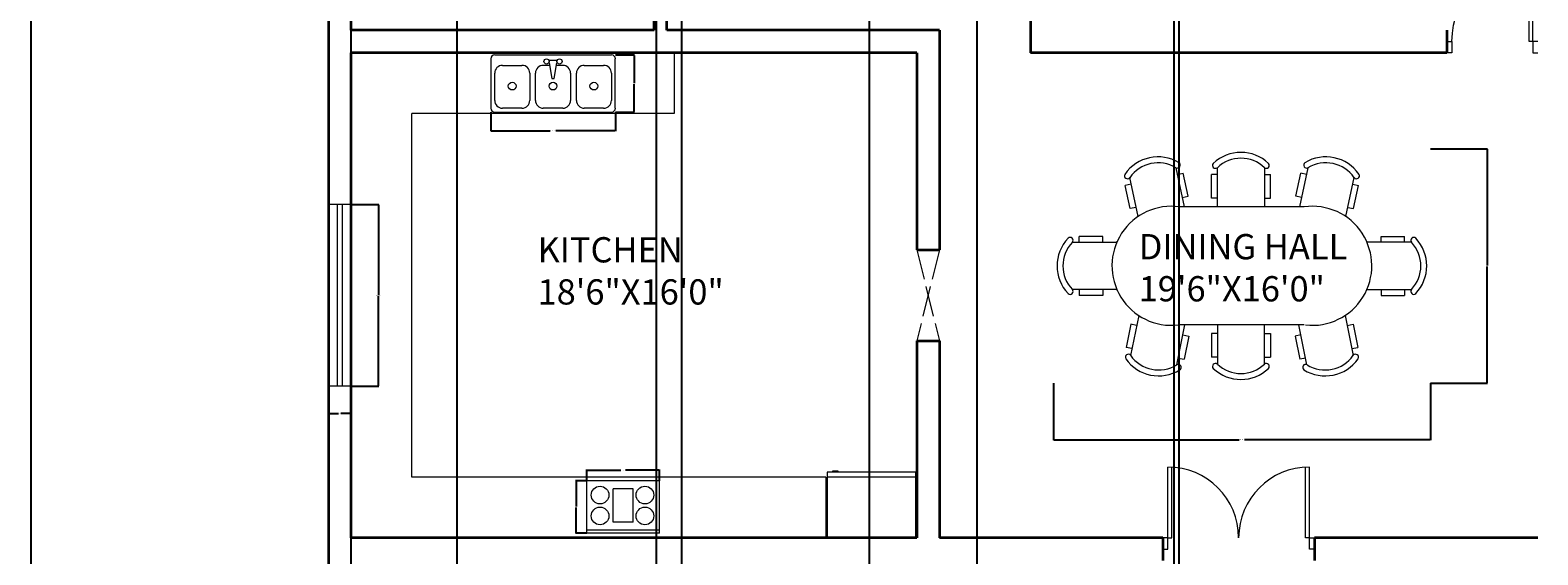
# Model space of a CAD drawing. Units: inches. Extents: x 4602 to 5612, y 5125 to 6591.
# Tile 4 of 6: x 4602 to 5199, y 5977 to 6185. Entities that reach past the tile are written whole.
import ezdxf

# ---------------------------------------------------------------- set-up
doc = ezdxf.new("R2010")
doc.units = ezdxf.units.IN
doc.linetypes.add('ACAD_ISO02W100', pattern=[15, 12, -3])
for name, color, linetype, lineweight in [('A-ANNO-DIMS', 2, 'Continuous', 18), ('A-AREA-IDEN', 7, 'Continuous', 18), ('A-DOOR', 4, 'Continuous', 18), ('A-EQPM', 8, 'Continuous', 18), ('A-FLOR-CASE', 9, 'Continuous', 18), ('A-FLOR-FIXT', 8, 'Continuous', 18), ('A-FURN', 8, 'Continuous', 13), ('A-GLAZ', 4, 'Continuous', 18), ('A-WALL', 7, 'Continuous', 35), ('A-WALL-OVHD', 8, 'ACAD_ISO02W100', 13)]:
    doc.layers.add(name, color=color, linetype=linetype, lineweight=lineweight)
doc.styles.get("Standard").update_dxf_attribs({"font": 'arial.ttf'})
doc.dimstyles.get("Standard").update_dxf_attribs({"dimtxt": 0.18, "dimasz": 0.18, "dimexe": 0.18, "dimexo": 0.0625, "dimgap": 0.09, "dimtad": 0, "dimtih": 1, "dimtoh": 1, "dimdec": 4, "dimzin": 0, "dimdsep": 46, "dimtxsty": 'Standard', "dimcen": 0.09, "dimadec": 0, "dimazin": 0, "dimtfac": 1, "dimtdec": 4, "dimtofl": 0, "dimtmove": 0, "dimatfit": 3, "dimfxl": 1, "dimtolj": 1, "dimtzin": 0, "dimarcsym": 0})

# ---------------------------------------------------------------- blocks, each defined once
blk = doc.blocks.new('A$C47C54457')
for p, q in [((0, 520), (720, 520)), ((0, 520), (0, 0)), ((0, 488), (720, 488)), ((720, 520), (720, 0)), ((262, 408), (458, 408)), ((262, 408), (262, 80)), ((458, 408), (458, 80)), ((0, 0), (720, 0)), ((262, 80), (458, 80))]:
    blk.add_line(p, q)
for centre in [(144, 348), (590, 348), (144, 140), (590, 140)]:
    blk.add_circle(centre, 88)
blk = doc.blocks.new('A$C4CC12AE8')
for p, q in [((1.006, 1.792), (1.077, 1.461)), ((1.357, 1.461), (1.357, 1.792)), ((1.757, 1.792), (1.757, 1.461)), ((2.124, 1.792), (2.053, 1.461)), ((0.686, 1.378), (0.615, 1.708)), ((1.018, 1.736), (1.067, 1.746)), ((1.109, 1.55), (1.067, 1.746)), ((1.357, 1.734), (1.307, 1.734)), ((1.307, 1.534), (1.307, 1.734)), ((1.757, 1.734), (1.807, 1.734)), ((1.807, 1.534), (1.807, 1.734)), ((2.022, 1.55), (2.063, 1.746)), ((2.112, 1.736), (2.063, 1.746)), ((2.445, 1.378), (2.515, 1.708)), ((0.627, 1.652), (0.578, 1.641)), ((0.62, 1.446), (0.578, 1.641)), ((1.06, 1.54), (1.109, 1.55)), ((1.357, 1.534), (1.307, 1.534)), ((1.757, 1.534), (1.807, 1.534)), ((2.07, 1.54), (2.022, 1.55)), ((2.503, 1.652), (2.552, 1.641)), ((2.51, 1.446), (2.552, 1.641)), ((0.669, 1.456), (0.62, 1.446)), ((2.093, 1.461), (1.038, 1.461)), ((2.462, 1.456), (2.51, 1.446)), ((0.13, 1.161), (0.5, 1.161)), ((0.188, 1.161), (0.188, 1.211)), ((0.388, 1.211), (0.188, 1.211)), ((0.388, 1.161), (0.388, 1.211)), ((3.001, 1.161), (2.631, 1.161)), ((2.743, 1.161), (2.743, 1.211)), ((2.743, 1.211), (2.943, 1.211)), ((2.943, 1.161), (2.943, 1.211)), ((0.5, 0.761), (0.13, 0.761)), ((0.188, 0.761), (0.188, 0.711)), ((0.388, 0.711), (0.188, 0.711)), ((0.388, 0.761), (0.388, 0.711)), ((2.631, 0.761), (3.001, 0.761)), ((2.743, 0.761), (2.743, 0.711)), ((2.743, 0.711), (2.943, 0.711)), ((2.943, 0.761), (2.943, 0.711)), ((0.691, 0.542), (0.622, 0.204)), ((2.439, 0.542), (2.508, 0.204)), ((0.625, 0.467), (0.585, 0.271)), ((0.674, 0.457), (0.625, 0.467)), ((1.014, 0.124), (1.083, 0.461)), ((2.093, 0.461), (1.038, 0.461)), ((1.357, 0.388), (1.307, 0.388)), ((1.307, 0.388), (1.307, 0.188)), ((1.357, 0.461), (1.357, 0.13)), ((1.757, 0.13), (1.757, 0.461)), ((1.757, 0.388), (1.807, 0.388)), ((1.807, 0.388), (1.807, 0.188)), ((2.116, 0.124), (2.048, 0.461)), ((2.457, 0.457), (2.506, 0.467)), ((2.506, 0.467), (2.546, 0.271)), ((0.634, 0.261), (0.585, 0.271)), ((1.066, 0.377), (1.115, 0.367)), ((1.115, 0.367), (1.075, 0.171)), ((2.065, 0.377), (2.016, 0.367)), ((2.016, 0.367), (2.056, 0.171)), ((2.497, 0.261), (2.546, 0.271)), ((1.026, 0.181), (1.075, 0.171)), ((1.357, 0.188), (1.307, 0.188)), ((1.757, 0.188), (1.807, 0.188)), ((2.105, 0.181), (2.056, 0.171))]:
    blk.add_line(p, q)
for centre, radius, start, end in [((1.557, 1.582), 0.34, 46.4394, 133.5606), ((0.855, 1.544), 0.34, 58.5263, 145.6476), ((0.855, 1.544), 0.29, 58.5263, 145.6476), ((1.017, 1.814), 0.0251, 243.3074, 53.7452), ((1.341, 1.812), 0.0251, 138.3417, 308.7795), ((1.557, 1.582), 0.29, 46.4394, 133.5606), ((1.772, 1.812), 0.0251, 231.2205, 41.6583), ((2.113, 1.814), 0.0251, 126.2548, 296.6926), ((2.276, 1.544), 0.34, 34.3524, 121.4737), ((2.276, 1.544), 0.29, 34.3524, 121.4737), ((0.596, 1.724), 0.0251, 150.4287, 320.8665), ((2.535, 1.724), 0.0251, 219.1335, 29.5713), ((0.969, 0.962), 0.504, 82.2325, 276.4385), ((2.161, 0.962), 0.504, 263.5615, 97.7675), ((0.34, 0.961), 0.34, 136.4394, 223.5606), ((0.34, 0.961), 0.29, 136.4394, 223.5606), ((0.11, 1.177), 0.0251, 321.2205, 131.6583), ((0.5, 1.131), 0.03, 77.6511, 90), ((2.631, 1.131), 0.03, 90, 102.3489), ((3.02, 1.177), 0.0251, 48.3417, 218.7795), ((2.79, 0.961), 0.29, 316.4394, 43.5606), ((2.79, 0.961), 0.34, 316.4394, 43.5606), ((0.11, 0.745), 0.0251, 228.3417, 38.7795), ((0.5, 0.791), 0.03, 270, 283.3086), ((2.631, 0.791), 0.03, 256.6914, 270), ((3.02, 0.745), 0.0251, 141.2205, 311.6583), ((0.603, 0.188), 0.0251, 39.6982, 210.136), ((0.86, 0.37), 0.34, 214.9171, 302.0384), ((0.86, 0.37), 0.29, 214.9171, 302.0384), ((1.341, 0.11), 0.0251, 51.2205, 221.6583), ((1.557, 0.34), 0.29, 226.4394, 313.5606), ((1.772, 0.11), 0.0251, 318.3417, 128.7795), ((2.27, 0.37), 0.34, 237.9616, 325.0829), ((2.27, 0.37), 0.29, 237.9616, 325.0829), ((2.527, 0.188), 0.0251, 329.864, 140.3018), ((1.026, 0.102), 0.0251, 306.8195, 117.2573), ((1.557, 0.34), 0.34, 226.4394, 313.5606), ((2.105, 0.102), 0.0251, 62.7427, 233.1805)]:
    blk.add_arc(centre, radius, start, end)
blk = doc.blocks.new('A$C762E1B96')
at = {"linetype": 'ByBlock'}
for p, q in [((0, 420), (0, 31)), ((952, 450), (31, 450)), ((92, 368), (246, 368)), ((464, 368), (414, 368)), ((460, 409), (522, 409)), ((460, 389), (481, 266)), ((501, 266), (522, 389)), ((568, 368), (518, 368)), ((737, 368), (890, 368)), ((982, 31), (982, 420)), ((31, 92), (31, 307)), ((307, 307), (307, 92)), ((353, 92), (353, 307)), ((481, 266), (501, 266)), ((629, 307), (629, 92)), ((675, 92), (675, 307)), ((952, 307), (952, 92)), ((246, 31), (92, 31)), ((568, 31), (414, 31)), ((890, 31), (737, 31)), ((31, 0), (952, 0))]:
    blk.add_line(p, q, dxfattribs=at)
for centre, radius in [((440, 399), 20.5), ((542, 399), 20.5), ((169, 205), 30.7), ((491, 205), 30.7), ((813, 205), 30.7)]:
    blk.add_circle(centre, radius, dxfattribs=at)
for centre, radius, start, end in [((31, 420), 30.7, 90, 180), ((92, 307), 61.4, 90, 180), ((246, 307), 61.4, 0, 90), ((414, 307), 61.4, 90, 180), ((568, 307), 61.4, 0, 90), ((737, 307), 61.4, 90, 180), ((890, 307), 61.4, 0, 90), ((952, 420), 30.7, 0, 90), ((31, 31), 30.7, 180, 270), ((92, 92), 61.4, 180, 270), ((246, 92), 61.4, 270, 0), ((414, 92), 61.4, 180, 270), ((568, 92), 61.4, 270, 0), ((737, 92), 61.4, 180, 270), ((890, 92), 61.4, 270, 0), ((952, 31), 30.7, 270, 0)]:
    blk.add_arc(centre, radius, start, end, dxfattribs=at)
at = {"flags": 9}
for tag in ['YSIZE', 'XSIZE']:
    blk.add_attdef(tag, (491, 450), '', height=0.5, rotation=270, dxfattribs=at)
blk = doc.blocks.new('DOOR-PAIR-60IN')
for p, q in [((2, 4.5), (2, 32.5)), ((3.5, 4.5), (3.5, 32.46)), ((56.5, 4.5), (56.5, 32.46)), ((58, 4.5), (58, 32.5)), ((2, 4.5), (0, 4.5)), ((2, 0), (2, 4.5)), ((2, 4.5), (3.5, 4.5)), ((58, 4.5), (56.5, 4.5)), ((58, 0), (58, 4.5)), ((58, 4.5), (60, 4.5)), ((0, 0), (2, 0)), ((60, 0), (58, 0))]:
    blk.add_line(p, q)
for centre, start, end in [((2, 4.5), 0, 90), ((58, 4.5), 90, 180)]:
    blk.add_arc(centre, 28, start, end)
blk = doc.blocks.new('DOOR-36IN-DEEP-JAMB')
for p, q in [((2, 4.5), (2, 36.5)), ((3.5, 4.5), (3.5, 36.46)), ((0, 4.5), (2, 4.5)), ((2, 4.5), (2, 0)), ((2, 4.5), (3.5, 4.5)), ((36, 4.5), (34, 4.5)), ((34, 4.5), (34, 0)), ((2, 0), (0, 0)), ((34, 0), (36, 0))]:
    blk.add_line(p, q)
blk.add_arc((2, 4.5), 32, 0, 90)
blk = doc.blocks.new('WINDOW-72IN')
for p, q in [((9, 72), (0, 72)), ((3.5, 72), (3.5, 0)), ((5.5, 72), (5.5, 0)), ((9, 0), (0, 0))]:
    blk.add_line(p, q)
blk = doc.blocks.new('*D31')
at = {"layer": 'A-ANNO-DIMS', "color": 0, "lineweight": -2, "transparency": 16777216}
for p, q in [((4729.3, 6115.55), (4740.22, 6115.55)), ((4740.04, 6115.37), (4740.04, 6079.73)), ((4740.04, 6043.73), (4740.04, 6079.37)), ((4729.3, 6043.55), (4740.22, 6043.55))]:
    blk.add_line(p, q, dxfattribs=at)
at = {"layer": 'A-ANNO-DIMS', "color": 0, "transparency": 16777216}
for points in [[(4740.01, 6115.37), (4740.07, 6115.37), (4740.04, 6115.55)], [(4740.01, 6043.73), (4740.07, 6043.73), (4740.04, 6043.55)]]:
    blk.add_solid(points, dxfattribs=at)
at = {"layer": 'Defpoints', "color": 0, "transparency": 16777216}
for p in [(4729.24, 6115.55), (4740.04, 6115.55), (4729.24, 6043.55)]:
    blk.add_point(p, dxfattribs=at)
at = {"layer": 'A-ANNO-DIMS', "color": 0, "transparency": 16777216, "insert": (4740.04, 6079.55), "char_height": 0.18, "attachment_point": 5}
blk.add_mtext('\\A1;WINDOW 72 TYP.', dxfattribs=at)
blk = doc.blocks.new('*D32')
at = {"layer": 'A-ANNO-DIMS', "color": 0, "lineweight": -2, "transparency": 16777216}
for p, q in [((4720.24, 6043.49), (4720.24, 6032.57)), ((4729.24, 6043.49), (4729.24, 6032.57)), ((4720.42, 6032.75), (4724.28, 6032.75)), ((4729.06, 6032.75), (4725.2, 6032.75))]:
    blk.add_line(p, q, dxfattribs=at)
at = {"layer": 'A-ANNO-DIMS', "color": 0, "transparency": 16777216}
for points in [[(4720.42, 6032.78), (4720.42, 6032.72), (4720.24, 6032.75)], [(4729.06, 6032.78), (4729.06, 6032.72), (4729.24, 6032.75)]]:
    blk.add_solid(points, dxfattribs=at)
at = {"layer": 'Defpoints', "color": 0, "transparency": 16777216}
for p in [(4720.24, 6043.55), (4729.24, 6043.55), (4729.24, 6032.75)]:
    blk.add_point(p, dxfattribs=at)
at = {"layer": 'A-ANNO-DIMS', "color": 0, "transparency": 16777216, "insert": (4724.74, 6032.75), "char_height": 0.18, "attachment_point": 5}
blk.add_mtext('\\A1;9 TYP.', dxfattribs=at)
blk = doc.blocks.new('*D45')
at = {"layer": 'A-ANNO-DIMS', "color": 0, "lineweight": -2, "transparency": 16777216}
for p, q in [((4822.63, 6006.13), (4822.63, 6010.55)), ((4822.81, 6010.37), (4836.11, 6010.37)), ((4851.16, 6010.37), (4837.87, 6010.37)), ((4851.34, 6006.13), (4851.34, 6010.55))]:
    blk.add_line(p, q, dxfattribs=at)
at = {"layer": 'A-ANNO-DIMS', "color": 0, "transparency": 16777216}
for points in [[(4822.81, 6010.4), (4822.81, 6010.34), (4822.63, 6010.37)], [(4851.16, 6010.4), (4851.16, 6010.34), (4851.34, 6010.37)]]:
    blk.add_solid(points, dxfattribs=at)
at = {"layer": 'Defpoints', "color": 0, "transparency": 16777216}
for p in [(4822.63, 6010.37), (4822.63, 6006.06), (4851.34, 6006.06)]:
    blk.add_point(p, dxfattribs=at)
at = {"layer": 'A-ANNO-DIMS', "color": 0, "transparency": 16777216, "insert": (4836.99, 6010.37), "char_height": 0.18, "attachment_point": 5}
blk.add_mtext('\\A1;COOKTOP 29', dxfattribs=at)
blk = doc.blocks.new('*D46')
at = {"layer": 'A-ANNO-DIMS', "color": 0, "lineweight": -2, "transparency": 16777216}
for p, q in [((4822.57, 6006.06), (4818.15, 6006.06)), ((4818.33, 6005.88), (4818.33, 5995.88)), ((4818.33, 5985.51), (4818.33, 5995.52)), ((4822.57, 5985.33), (4818.15, 5985.33))]:
    blk.add_line(p, q, dxfattribs=at)
at = {"layer": 'A-ANNO-DIMS', "color": 0, "transparency": 16777216}
for points in [[(4818.3, 6005.88), (4818.36, 6005.88), (4818.33, 6006.06)], [(4818.3, 5985.51), (4818.36, 5985.51), (4818.33, 5985.33)]]:
    blk.add_solid(points, dxfattribs=at)
at = {"layer": 'Defpoints', "color": 0, "transparency": 16777216}
for p in [(4822.63, 6006.06), (4818.33, 5985.33), (4822.63, 5985.33)]:
    blk.add_point(p, dxfattribs=at)
at = {"layer": 'A-ANNO-DIMS', "color": 0, "transparency": 16777216, "insert": (4818.33, 5995.7), "char_height": 0.18, "attachment_point": 5}
blk.add_mtext('\\A1;21', dxfattribs=at)
blk = doc.blocks.new('*D47')
at = {"layer": 'A-ANNO-DIMS', "color": 0, "lineweight": -2, "transparency": 16777216}
for p, q in [((5007.36, 6044.73), (5007.36, 6022.21)), ((5156.72, 6044.73), (5156.72, 6022.21)), ((5007.54, 6022.39), (5081, 6022.39)), ((5156.54, 6022.39), (5083.08, 6022.39))]:
    blk.add_line(p, q, dxfattribs=at)
at = {"layer": 'A-ANNO-DIMS', "color": 0, "transparency": 16777216}
for points in [[(5007.54, 6022.42), (5007.54, 6022.36), (5007.36, 6022.39)], [(5156.54, 6022.42), (5156.54, 6022.36), (5156.72, 6022.39)]]:
    blk.add_solid(points, dxfattribs=at)
at = {"layer": 'Defpoints', "color": 0, "transparency": 16777216}
for p in [(5007.36, 6044.79), (5156.72, 6044.79), (5156.72, 6022.39)]:
    blk.add_point(p, dxfattribs=at)
at = {"layer": 'A-ANNO-DIMS', "color": 0, "transparency": 16777216, "insert": (5082.04, 6022.39), "char_height": 0.18, "attachment_point": 5}
blk.add_mtext('\\A1;DINING SET 149', dxfattribs=at)
blk = doc.blocks.new('*D48')
at = {"layer": 'A-ANNO-DIMS', "color": 0, "lineweight": -2, "transparency": 16777216}
for p, q in [((5156.78, 6137.62), (5179.3, 6137.62)), ((5179.12, 6137.44), (5179.12, 6091.39)), ((5179.12, 6044.97), (5179.12, 6091.02)), ((5156.78, 6044.79), (5179.3, 6044.79))]:
    blk.add_line(p, q, dxfattribs=at)
at = {"layer": 'A-ANNO-DIMS', "color": 0, "transparency": 16777216}
for points in [[(5179.09, 6137.44), (5179.15, 6137.44), (5179.12, 6137.62)], [(5179.09, 6044.97), (5179.15, 6044.97), (5179.12, 6044.79)]]:
    blk.add_solid(points, dxfattribs=at)
at = {"layer": 'Defpoints', "color": 0, "transparency": 16777216}
for p in [(5156.72, 6137.62), (5179.12, 6137.62), (5156.72, 6044.79)]:
    blk.add_point(p, dxfattribs=at)
at = {"layer": 'A-ANNO-DIMS', "color": 0, "transparency": 16777216, "insert": (5179.12, 6091.21), "char_height": 0.18, "attachment_point": 5}
blk.add_mtext('\\A1;93', dxfattribs=at)
blk = doc.blocks.new('*D53')
at = {"layer": 'A-ANNO-DIMS', "color": 0, "lineweight": -2, "transparency": 16777216}
for p, q in [((4784.55, 6152.05), (4784.55, 6144.53)), ((4833.89, 6152.05), (4833.89, 6144.53)), ((4784.73, 6144.71), (4808.09, 6144.71)), ((4833.71, 6144.71), (4810.35, 6144.71))]:
    blk.add_line(p, q, dxfattribs=at)
at = {"layer": 'A-ANNO-DIMS', "color": 0, "transparency": 16777216}
for points in [[(4784.73, 6144.74), (4784.73, 6144.68), (4784.55, 6144.71)], [(4833.71, 6144.74), (4833.71, 6144.68), (4833.89, 6144.71)]]:
    blk.add_solid(points, dxfattribs=at)
at = {"layer": 'Defpoints', "color": 0, "transparency": 16777216}
for p in [(4784.55, 6152.11), (4833.89, 6152.11), (4833.89, 6144.71)]:
    blk.add_point(p, dxfattribs=at)
at = {"layer": 'A-ANNO-DIMS', "color": 0, "transparency": 16777216, "insert": (4809.22, 6144.71), "char_height": 0.18, "attachment_point": 5}
blk.add_mtext('\\A1;KITCHEN SINK 49', dxfattribs=at)
blk = doc.blocks.new('*D54')
at = {"layer": 'A-ANNO-DIMS', "color": 0, "lineweight": -2, "transparency": 16777216}
for p, q in [((4833.95, 6174.72), (4841.47, 6174.72)), ((4841.29, 6174.54), (4841.29, 6163.6)), ((4841.29, 6152.29), (4841.29, 6163.23)), ((4833.95, 6152.11), (4841.47, 6152.11))]:
    blk.add_line(p, q, dxfattribs=at)
at = {"layer": 'A-ANNO-DIMS', "color": 0, "transparency": 16777216}
for points in [[(4841.26, 6174.54), (4841.32, 6174.54), (4841.29, 6174.72)], [(4841.26, 6152.29), (4841.32, 6152.29), (4841.29, 6152.11)]]:
    blk.add_solid(points, dxfattribs=at)
at = {"layer": 'Defpoints', "color": 0, "transparency": 16777216}
for p in [(4833.89, 6174.72), (4841.29, 6174.72), (4833.89, 6152.11)]:
    blk.add_point(p, dxfattribs=at)
at = {"layer": 'A-ANNO-DIMS', "color": 0, "transparency": 16777216, "insert": (4841.29, 6163.41), "char_height": 0.18, "attachment_point": 5}
blk.add_mtext('\\A1;23', dxfattribs=at)
blk = doc.blocks.new('*D55')
at = {"layer": 'A-ANNO-DIMS', "color": 0, "lineweight": -2, "transparency": 16777216}
for p, q in [((4674.24, 6252.95), (4674.24, 6572.85)), ((4674.42, 6572.67), (5106.95, 6572.67)), ((5540.06, 6572.67), (5107.53, 6572.67)), ((5540.24, 6127.61), (5540.24, 6572.85))]:
    blk.add_line(p, q, dxfattribs=at)
at = {"layer": 'A-ANNO-DIMS', "color": 0, "transparency": 16777216}
for points in [[(4674.42, 6572.7), (4674.42, 6572.64), (4674.24, 6572.67)], [(5540.06, 6572.7), (5540.06, 6572.64), (5540.24, 6572.67)]]:
    blk.add_solid(points, dxfattribs=at)
at = {"layer": 'Defpoints', "color": 0, "transparency": 16777216}
for p in [(5540.24, 6572.67), (4674.24, 6252.89), (5540.24, 6127.55)]:
    blk.add_point(p, dxfattribs=at)
at = {"layer": 'A-ANNO-DIMS', "color": 0, "transparency": 16777216, "insert": (5107.24, 6572.67), "char_height": 0.18, "attachment_point": 5}
blk.add_mtext('\\A1;866', dxfattribs=at)
blk = doc.blocks.new('*D56')
at = {"layer": 'A-ANNO-DIMS', "color": 0, "lineweight": -2, "transparency": 16777216}
for p, q in [((5061.18, 6438.55), (4602.21, 6438.55)), ((4602.39, 6438.37), (4602.39, 5817.73)), ((4602.39, 5196.73), (4602.39, 5817.37)), ((5055.18, 5196.55), (4602.21, 5196.55))]:
    blk.add_line(p, q, dxfattribs=at)
at = {"layer": 'A-ANNO-DIMS', "color": 0, "transparency": 16777216}
for points in [[(4602.36, 6438.37), (4602.42, 6438.37), (4602.39, 6438.55)], [(4602.36, 5196.73), (4602.42, 5196.73), (4602.39, 5196.55)]]:
    blk.add_solid(points, dxfattribs=at)
at = {"layer": 'Defpoints', "color": 0, "transparency": 16777216}
for p in [(4602.39, 6438.55), (5061.24, 6438.55), (5055.24, 5196.55)]:
    blk.add_point(p, dxfattribs=at)
at = {"layer": 'A-ANNO-DIMS', "color": 0, "transparency": 16777216, "insert": (4602.39, 5817.55), "char_height": 0.18, "attachment_point": 5}
blk.add_mtext('\\A1;1242', dxfattribs=at)
blk = doc.blocks.new('*D59')
at = {"layer": 'A-ANNO-DIMS', "color": 0, "lineweight": -2, "transparency": 16777216}
for p, q in [((4977.24, 5908.61), (4977.24, 6572.85)), ((4977.42, 6572.67), (5016.82, 6572.67)), ((5056.97, 6572.67), (5017.57, 6572.67)), ((5057.15, 5908.61), (5057.15, 6572.85))]:
    blk.add_line(p, q, dxfattribs=at)
at = {"layer": 'A-ANNO-DIMS', "color": 0, "transparency": 16777216}
for points in [[(4977.42, 6572.7), (4977.42, 6572.64), (4977.24, 6572.67)], [(5056.97, 6572.7), (5056.97, 6572.64), (5057.15, 6572.67)]]:
    blk.add_solid(points, dxfattribs=at)
at = {"layer": 'Defpoints', "color": 0, "transparency": 16777216}
for p in [(5057.15, 6572.67), (4977.24, 5908.55), (5057.15, 5908.55)]:
    blk.add_point(p, dxfattribs=at)
at = {"layer": 'A-ANNO-DIMS', "color": 0, "transparency": 16777216, "insert": (5017.19, 6572.67), "char_height": 0.18, "attachment_point": 5}
blk.add_mtext('\\A1;79.91', dxfattribs=at)
blk = doc.blocks.new('*D60')
at = {"layer": 'A-ANNO-DIMS', "color": 0, "lineweight": -2, "transparency": 16777216}
for p, q in [((4934.59, 5248.61), (4934.59, 6572.85)), ((4934.77, 6572.67), (4994.46, 6572.67)), ((5055.06, 6572.67), (4995.37, 6572.67)), ((5055.24, 5248.61), (5055.24, 6572.85))]:
    blk.add_line(p, q, dxfattribs=at)
at = {"layer": 'A-ANNO-DIMS', "color": 0, "transparency": 16777216}
for points in [[(4934.77, 6572.7), (4934.77, 6572.64), (4934.59, 6572.67)], [(5055.06, 6572.7), (5055.06, 6572.64), (5055.24, 6572.67)]]:
    blk.add_solid(points, dxfattribs=at)
at = {"layer": 'Defpoints', "color": 0, "transparency": 16777216}
for p in [(5055.24, 6572.67), (4934.59, 5248.55), (5055.24, 5248.55)]:
    blk.add_point(p, dxfattribs=at)
at = {"layer": 'A-ANNO-DIMS', "color": 0, "transparency": 16777216, "insert": (4994.91, 6572.67), "char_height": 0.18, "attachment_point": 5}
blk.add_mtext('\\A1;120.65', dxfattribs=at)
blk = doc.blocks.new('*D62')
at = {"layer": 'A-ANNO-DIMS', "color": 0, "lineweight": -2, "transparency": 16777216}
for p, q in [((4729.24, 5886.61), (4729.24, 6572.85)), ((4729.42, 6572.67), (4750.02, 6572.67)), ((4771.06, 6572.67), (4750.46, 6572.67)), ((4771.24, 5886.61), (4771.24, 6572.85))]:
    blk.add_line(p, q, dxfattribs=at)
at = {"layer": 'A-ANNO-DIMS', "color": 0, "transparency": 16777216}
for points in [[(4729.42, 6572.7), (4729.42, 6572.64), (4729.24, 6572.67)], [(4771.06, 6572.7), (4771.06, 6572.64), (4771.24, 6572.67)]]:
    blk.add_solid(points, dxfattribs=at)
at = {"layer": 'Defpoints', "color": 0, "transparency": 16777216}
for p in [(4771.24, 6572.67), (4729.24, 5886.55), (4771.24, 5886.55)]:
    blk.add_point(p, dxfattribs=at)
at = {"layer": 'A-ANNO-DIMS', "color": 0, "transparency": 16777216, "insert": (4750.24, 6572.67), "char_height": 0.18, "attachment_point": 5}
blk.add_mtext('\\A1;42', dxfattribs=at)
blk = doc.blocks.new('*D63')
at = {"layer": 'A-ANNO-DIMS', "color": 0, "lineweight": -2, "transparency": 16777216}
for p, q in [((4850.24, 5876.61), (4850.24, 6572.85)), ((4850.42, 6572.67), (4855.03, 6572.67)), ((4860.06, 6572.67), (4855.45, 6572.67)), ((4860.24, 5876.61), (4860.24, 6572.85))]:
    blk.add_line(p, q, dxfattribs=at)
at = {"layer": 'A-ANNO-DIMS', "color": 0, "transparency": 16777216}
for points in [[(4850.42, 6572.7), (4850.42, 6572.64), (4850.24, 6572.67)], [(4860.06, 6572.7), (4860.06, 6572.64), (4860.24, 6572.67)]]:
    blk.add_solid(points, dxfattribs=at)
at = {"layer": 'Defpoints', "color": 0, "transparency": 16777216}
for p in [(4860.24, 6572.67), (4850.24, 5876.55), (4860.24, 5876.55)]:
    blk.add_point(p, dxfattribs=at)
at = {"layer": 'A-ANNO-DIMS', "color": 0, "transparency": 16777216, "insert": (4855.24, 6572.67), "char_height": 0.18, "attachment_point": 5}
blk.add_mtext('\\A1;10', dxfattribs=at)

msp = doc.modelspace()

# ---------------------------------------------------------------- linework, layer by layer
at = {"layer": 'A-EQPM'}
for p, q in [((4917.739, 6009.5515), (4917.739, 5983.5515)), ((4952.739, 6009.5515), (4917.739, 6009.5515)), ((4952.739, 6007.5515), (4917.739, 6007.5515)), ((4920.0391, 6009.5515), (4920.0391, 6010.0946)), ((4920.0391, 6010.0946), (4922.0391, 6010.0946)), ((4922.0391, 6010.0946), (4922.0391, 6009.5515)), ((4952.739, 6009.5515), (4952.739, 5983.5515))]:
    msp.add_line(p, q, dxfattribs=at)
at = {"layer": 'A-FLOR-CASE'}
for p, q in [((4857.239, 6175.5515), (4857.239, 6151.5515)), ((4753.239, 6007.5515), (4753.239, 6151.5515)), ((4857.239, 6151.5515), (4753.239, 6151.5515)), ((4917.239, 6007.5515), (4753.239, 6007.5515)), ((4917.239, 6007.5515), (4917.239, 5983.5515))]:
    msp.add_line(p, q, dxfattribs=at)
at = {"layer": 'A-WALL'}
for p, q in [((4998.239, 6304.5515), (4998.239, 6175.5515)), ((4849.239, 6184.5515), (4849.239, 6226.5515)), ((4854.239, 6184.5515), (4854.239, 6226.5515)), ((4720.239, 6208.5515), (4720.239, 5380.5515)), ((4729.239, 6184.5515), (4729.239, 6208.5515)), ((4849.239, 6184.5515), (4729.239, 6184.5515)), ((4962.239, 6184.5515), (4854.239, 6184.5515)), ((4962.239, 6184.5515), (4962.239, 6175.5515)), ((5163.239, 6184.5515), (5163.239, 6175.5515)), ((4729.239, 5983.5515), (4729.239, 6175.5515)), ((4953.239, 6175.5515), (4729.239, 6175.5515)), ((4953.239, 6175.5515), (4953.239, 6097.5515)), ((4962.239, 6175.5515), (4962.239, 6097.5515)), ((5163.239, 6175.5515), (4998.239, 6175.5515)), ((4953.239, 6097.5515), (4962.239, 6097.5515)), ((4953.239, 6061.5515), (4962.239, 6061.5515)), ((4953.239, 6061.5515), (4953.239, 5983.5515)), ((4962.239, 6061.5515), (4962.239, 5983.5515)), ((4953.239, 5983.5515), (4729.239, 5983.5515)), ((5050.739, 5983.5515), (4962.239, 5983.5515)), ((5050.739, 5983.5515), (5050.739, 5974.5515)), ((5199.239, 5983.5515), (5110.739, 5983.5515)), ((5110.739, 5983.5515), (5110.739, 5974.5515))]:
    msp.add_line(p, q, dxfattribs=at)
at = {"layer": 'A-WALL-OVHD'}
for p, q in [((4962.239, 6097.5515), (4953.239, 6061.5515)), ((4953.239, 6097.5515), (4962.239, 6061.5515))]:
    msp.add_line(p, q, dxfattribs=at)

# ---------------------------------------------------------------- block references
at = {"layer": 'A-DOOR', "extrusion": (0, 0, -1), "zscale": -1}
msp.add_blockref('DOOR-36IN-DEEP-JAMB', (-5199.2391, 6175.552), dxfattribs=at)
at = {"layer": 'A-DOOR'}
msp.add_blockref('DOOR-PAIR-60IN', (5050.739, 5979.052), dxfattribs=at)
at = {"layer": 'A-EQPM', "xscale": 0.0398727721898774, "yscale": 0.0398727721898774, "zscale": 0.0398727721898774, "rotation": 180}
msp.add_blockref('A$C47C54457', (4851.3425, 6006.0635), dxfattribs=at)
at = {"layer": 'A-FLOR-FIXT', "xscale": 0.0502260172947709, "yscale": 0.0502260172947709, "zscale": 0.0502260172947709}
msp.add_blockref('A$C762E1B96', (4784.552, 6152.1082), dxfattribs=at)
at = {"layer": 'A-FURN', "xscale": 46.77888076022151, "yscale": 46.77888076022151, "zscale": 46.77888076022151}
msp.add_blockref('A$C4CC12AE8', (5008.8209, 6046.2541), dxfattribs=at)
at = {"layer": 'A-GLAZ'}
msp.add_blockref('WINDOW-72IN', (4720.239, 6043.552), dxfattribs=at)

# ---------------------------------------------------------------- texts
at = {"layer": 'A-AREA-IDEN', "char_height": 10, "attachment_point": 1}
for s, width, insert in [('KITCHEN\\P18\'6"X16\'0"', 140.595401, (4803.0688, 6102.5794)), ('DINING HALL\\P19\'6"X16\'0"', 326.752228, (5041.1571, 6103.8221))]:
    msp.add_mtext_dynamic_manual_height_columns(s, width=width, gutter_width=12.5, heights=[0], dxfattribs=dict(at, insert=insert))

# ---------------------------------------------------------------- dimensions: what is measured, and where the dimension line sits
at = {"layer": 'A-ANNO-DIMS'}
for base, p1, p2, override, picture, middle in [((5540.239, 6572.6716), (4674.239, 6252.8852), (5540.239, 6127.5515), {"dimdec": 0, "dimlfac": 1, "dimrnd": 0, "dimzin": 0, "dimdsep": 46, "dimlunit": 2}, '*D55', (5107.239, 6572.6716)), ((4771.239, 6572.6716), (4729.239, 5886.5515), (4771.239, 5886.5515), {"dimdec": 0, "dimlfac": 1, "dimrnd": 0, "dimzin": 0, "dimdsep": 46, "dimlunit": 2}, '*D62', (4750.239, 6572.6716)), ((4860.239, 6572.6716), (4850.239, 5876.5515), (4860.239, 5876.5515), {"dimdec": 0, "dimlfac": 1, "dimrnd": 0, "dimzin": 0, "dimdsep": 46, "dimlunit": 2}, '*D63', (4855.239, 6572.6716)), ((5055.239, 6572.6716), (4934.5878, 5248.5515), (5055.239, 5248.5515), {"dimdec": 2, "dimlfac": 1, "dimrnd": 0, "dimzin": 0, "dimdsep": 46, "dimlunit": 2}, '*D60', (4994.9134, 6572.6716)), ((5057.1497, 6572.6716), (4977.239, 5908.5515), (5057.1497, 5908.5515), {"dimdec": 2, "dimlfac": 1, "dimrnd": 0, "dimzin": 0, "dimdsep": 46, "dimlunit": 2}, '*D59', (5017.1944, 6572.6716))]:
    dim = msp.add_linear_dim(base=base, p1=p1, p2=p2, dimstyle='Standard', override=override, dxfattribs=at)
    dim.commit()
    dim.dimension.update_dxf_attribs({"geometry": picture, "text_midpoint": middle})
for base, p1, p2, angle, picture, middle in [((4602.389, 6438.5515), (5055.239, 5196.5515), (5061.239, 6438.5515), 90, '*D56', (4602.389, 5817.5515)), ((4841.2869, 6174.7199), (4833.8867, 6152.1082), (4833.8867, 6174.7199), 90, '*D54', (4841.2869, 6163.4141)), ((5179.1247, 6137.6173), (5156.7206, 6044.7934), (5156.7206, 6137.6173), 90, '*D48', (5179.1247, 6091.2053)), ((4818.3278, 5985.3296), (4822.6341, 6006.0635), (4822.6341, 5985.3296), 270, '*D46', (4818.3278, 5995.6965))]:
    dim = msp.add_linear_dim(base=base, p1=p1, p2=p2, angle=angle, dimstyle='Standard', override={"dimdec": 0, "dimlfac": 1, "dimrnd": 0, "dimzin": 0, "dimdsep": 46, "dimlunit": 2}, dxfattribs=at)
    dim.commit()
    dim.dimension.update_dxf_attribs({"geometry": picture, "text_midpoint": middle})
for base, p1, p2, text, picture, middle in [((4833.8867, 6144.708), (4784.552, 6152.1082), (4833.8867, 6152.1082), 'KITCHEN SINK <>', '*D53', (4809.2193, 6144.708)), ((4729.239, 6032.7515), (4720.239, 6043.5515), (4729.239, 6043.5515), '<> TYP.', '*D32', (4724.739, 6032.7515)), ((5156.7206, 6022.3893), (5007.3601, 6044.7934), (5156.7206, 6044.7934), 'DINING SET <>', '*D47', (5082.0404, 6022.3893))]:
    dim = msp.add_linear_dim(base=base, p1=p1, p2=p2, text=text, dimstyle='Standard', override={"dimdec": 0, "dimlfac": 1, "dimrnd": 0, "dimzin": 0, "dimdsep": 46, "dimlunit": 2}, dxfattribs=at)
    dim.commit()
    dim.dimension.update_dxf_attribs({"geometry": picture, "text_midpoint": middle})
for base, p1, p2, angle, text, picture, middle in [((4740.039, 6115.5515), (4729.239, 6043.5515), (4729.239, 6115.5515), 90, 'WINDOW <> TYP.', '*D31', (4740.039, 6079.5515)), ((4822.6341, 6010.3697), (4851.3425, 6006.0635), (4822.6341, 6006.0635), 180, 'COOKTOP <>', '*D45', (4836.9883, 6010.3697))]:
    dim = msp.add_linear_dim(base=base, p1=p1, p2=p2, angle=angle, text=text, dimstyle='Standard', override={"dimdec": 0, "dimlfac": 1, "dimrnd": 0, "dimzin": 0, "dimdsep": 46, "dimlunit": 2}, dxfattribs=at)
    dim.commit()
    dim.dimension.update_dxf_attribs({"geometry": picture, "text_midpoint": middle})

doc.saveas('drawing.dxf')
